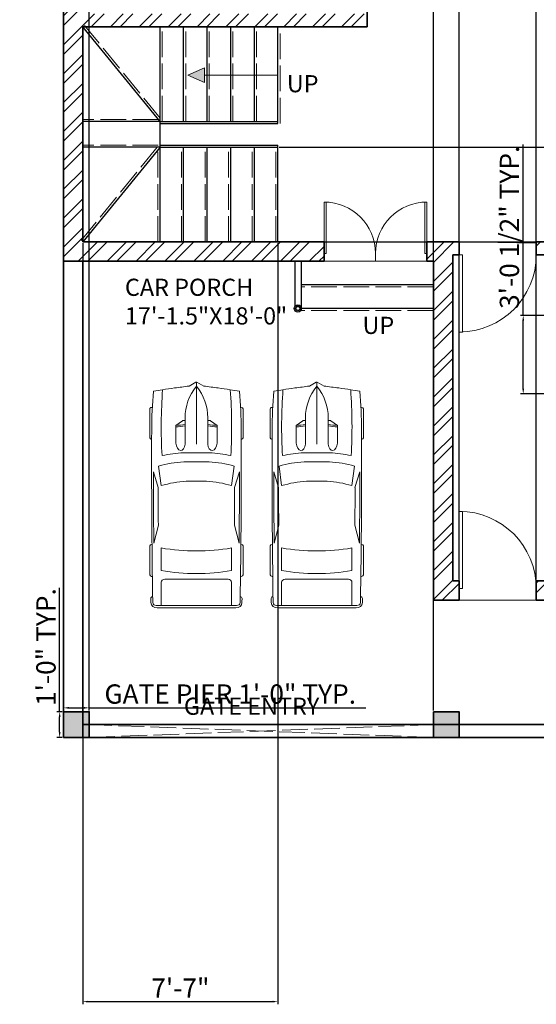
# Model space of a CAD drawing. Units: inches. Extents: x 744 to 1448, y 5126 to 6077.
# Tile 1 of 10: x 784 to 1025, y 5126 to 5585. Entities that reach past the tile are written whole.
import ezdxf

# ---------------------------------------------------------------- set-up
doc = ezdxf.new("R2010")
doc.units = ezdxf.units.IN
doc.linetypes.add('ACAD_ISO02W100', pattern=[15, 12, -3])
for name, color, linetype, lineweight in [('A-ANNO-DIMS', 2, 'Continuous', 18), ('A-ANNO-SYMB', 7, 'Continuous', 18), ('A-ANNO-TEXT', 7, 'Continuous', 18), ('A-AREA-IDEN', 7, 'Continuous', 18), ('A-COLS', 7, 'Continuous', 35), ('A-DOOR', 4, 'Continuous', 18), ('A-FLOR-STRS', 7, 'Continuous', 25), ('A-FLOR-STRS-HIDN', 8, 'ACAD_ISO02W100', 13), ('A-SITE-VEHI', 8, 'Continuous', 13), ('A-WALL', 7, 'Continuous', 35), ('A-WALL-PATT', 252, 'Continuous', 13)]:
    doc.layers.add(name, color=color, linetype=linetype, lineweight=lineweight)
doc.layers.add('A-SITE-GATE', color=244, linetype='ACAD_ISO02W100', lineweight=13, true_color=0x991b1e)
doc.styles.get("Standard").update_dxf_attribs({"font": 'arial.ttf'})
doc.dimstyles.new('ISO-25', dxfattribs={"dimtxt": 9, "dimasz": 2.5, "dimexe": 1.25, "dimexo": 0.625, "dimtad": 1, "dimlunit": 3, "dimtxsty": 'Standard', "dimcen": 2.5, "dimadec": 0, "dimazin": 0, "dimtfac": 1, "dimtmove": 0, "dimatfit": 3, "dimfxl": 1, "dimarcsym": 0})

# ---------------------------------------------------------------- blocks, each defined once
blk = doc.blocks.new('*U5')
for p, q in [((0, 0), (0, 6)), ((40, 0), (40, 6))]:
    blk.add_line(p, q)
blk.add_lwpolyline([(0, 0), (0, -40), (1.75, -40), (1.75, 0)], close=True)
blk.add_arc((0, 0), 40, 270, 0)
blk = doc.blocks.new('*U2')
for p, q in [((0, 0), (0, -6)), ((40, 0), (40, -6))]:
    blk.add_line(p, q)
blk.add_lwpolyline([(0, 0), (0, 40), (1.75, 40), (1.75, 0)], close=True)
blk.add_arc((0, 0), 40, 0, 90)
blk = doc.blocks.new('*U6')
for p, q in [((0, 0), (0, -6)), ((-40, 0), (-40, -6))]:
    blk.add_line(p, q)
blk.add_lwpolyline([(0, 0), (0, 40), (-1.75, 40), (-1.75, 0)], close=True)
blk.add_arc((0, 0), 40, 90, 180)
blk = doc.blocks.new('*U22')
for p, q in [((21.1, 37.41), (21.1, 36.83)), ((46.55, 38.89), (22.35, 38.89)), ((47.8, 37.39), (47.8, 37.41)), ((87.99, 31.87), (74.76, 35.92)), ((134.31, 35.6), (119.29, 31.78)), ((135.45, 37.07), (135.45, 37.41)), ((136.7, 38.89), (160.9, 38.89)), ((162.15, 37.41), (162.15, 36.77)), ((186.47, -33.5), (186.47, 33.5)), ((70.03, 31.54), (86.41, 29.35)), ((138.42, 29.35), (157.25, 29.35)), ((164.52, 26.39), (164.52, -26.39)), ((186.47, 29.35), (167.01, 29.35)), ((188.4, -32.76), (188.4, 32.76)), ((32.27, 11.63), (36.13, 17.17)), ((36.13, 17.17), (50.94, 17.17)), ((29.77, 9.51), (51.68, 9.51)), ((32.12, 9.51), (32.12, 11.15)), ((58.92, -10.77), (58.92, 10.77)), ((66.55, -10.53), (66.55, 10.53)), ((82.74, 8.5), (82.74, -8.5)), ((186.47, -10.53), (186.47, 10.53)), ((3.27, 6.13), (0.1, 0.41)), ((0, 0), (51.68, 0)), ((0.1, -0.41), (3.27, -6.13)), ((29.77, -9.51), (51.68, -9.51)), ((32.12, -9.51), (32.12, -11.15)), ((32.27, -11.63), (36.13, -17.17)), ((36.13, -17.17), (50.94, -17.17)), ((86.41, -29.35), (70.03, -31.54)), ((87.99, -31.87), (74.76, -35.92)), ((134.31, -35.6), (119.29, -31.78)), ((157.25, -29.35), (138.42, -29.35)), ((167.01, -29.35), (186.47, -29.35)), ((21.1, -37.41), (21.1, -36.83)), ((46.55, -38.89), (22.35, -38.89)), ((47.8, -37.39), (47.8, -37.41)), ((135.45, -37.07), (135.45, -37.41)), ((136.7, -38.89), (160.9, -38.89)), ((162.15, -37.41), (162.15, -36.77))]:
    blk.add_line(p, q)
for centre, major_axis, ratio, start_param, end_param in [((266.03, -27.52), (0, 313.31), 0.842304, 1.367076, 1.39176), ((41.19, -490.86), (0, 528.23), 0.842304, 0.00281, 0.075598), ((22.35, 37.41), (0, -1.48), 0.842304, 3.141593, 4.712389), ((64.48, -10555.62), (0, 10593.03), 0.842304, -0.013397, 0.002797), ((46.55, 37.41), (0, 1.48), 0.842304, -1.570796, 0), ((64.48, -10555.62), (0, -10591.55), 0.842304, 3.133765, 3.140441), ((136.7, 37.41), (0, -1.48), 0.842304, 3.141593, 4.712389), ((160.9, 37.41), (0, 1.48), 0.842304, -1.570796, 0), ((180.63, 35.84), (0, 2.22), 0.842304, -0.013017, 1.249894), ((64.48, -10556.36), (0, 10595.31), 0.842304, -0.013397, -0.013017), ((183.98, 33.5), (0, -2.96), 0.842304, 1.570796, 3.128196), ((183.98, 32.76), (0, -5.25), 0.842304, 1.570796, 3.128196), ((259.18, -27.52), (0, -305.3), 0.842304, 4.528606, 4.561838), ((37.47, -593.96), (0, -623.33), 0.842304, 3.096046, 3.200911), ((134.4, 5.39), (0, -89.78), 0.842304, 4.449482, 4.652344), ((135.29, 5.39), (0, 81.77), 0.842304, 1.245306, 1.50788), ((149.6, 2.8), (0, -79.58), 0.842304, 4.372215, 4.640744), ((95.79, -3666.35), (0, -3698.24), 0.842304, 3.134049, 3.144098), ((17.08, 0), (0, 147.02), 0.842304, 4.511394, 4.913384), ((35.91, 0), (0, 147.02), 0.842304, 4.511394, 4.913384), ((167.01, 26.39), (0, 2.96), 0.842304, 0, 1.570796), ((-204.49, 52.4), (0, -250.96), 0.842304, 1.385369, 1.434372), ((13.04, 17.01), (0, 27.42), 0.842304, 4.435146, 4.718221), ((14.2, 17.01), (0, 27.42), 0.842304, 4.435146, 4.718221), ((50.79, 13.34), (6.34, -0.36), 0.603834, -1.395552, 1.581315), ((29.77, -46.66), (0, 56.17), 0.842304, 0, 0.590319), ((32.75, 11.15), (0, 0.74), 0.842304, 0.879714, 1.570796), ((0.62, 0), (0, -0.74), 0.842304, 4.131459, 5.293319), ((-204.49, -52.4), (0, 250.96), 0.842304, -1.434372, -1.385369), ((29.77, 46.66), (0, 56.17), 0.842304, 2.551274, 3.141593), ((32.75, -11.15), (0, -0.74), 0.842304, 4.712389, 5.403472), ((13.04, -17.01), (0, -27.42), 0.842304, 1.564964, 1.848039), ((14.2, -17.01), (0, -27.42), 0.842304, 1.564964, 1.848039), ((134.4, -5.39), (0, -89.78), 0.842304, -1.510751, -1.307889), ((135.29, -5.39), (0, -81.77), 0.842304, -1.50788, -1.245306), ((149.6, -2.8), (0, -79.58), 0.842304, -1.499151, -1.230623), ((259.18, 27.52), (0, 305.3), 0.842304, 1.721348, 1.754579), ((266.03, 27.52), (0, 313.31), 0.842304, 1.749832, 1.774517), ((37.47, 593.96), (0, -623.33), 0.842304, -0.059319, 0.045547), ((95.79, 3666.35), (0, -3698.24), 0.842304, -0.002505, 0.007544), ((167.01, -26.39), (0, -2.96), 0.842304, 4.712389, 6.283185), ((183.98, -32.76), (0, -5.25), 0.842304, 0.013397, 1.570796), ((41.19, 490.86), (0, -528.23), 0.842304, -0.075598, -0.00281), ((22.35, -37.41), (0, 1.48), 0.842304, 1.570796, 3.141593), ((64.48, 10555.62), (0, 10593.03), 0.842304, 3.138796, 3.15499), ((46.55, -37.41), (0, -1.48), 0.842304, 0, 1.570796), ((64.48, 10555.62), (0, -10591.55), 0.842304, 0.001152, 0.007828), ((136.7, -37.41), (0, -1.48), 0.842304, -1.570796, 0), ((160.9, -37.41), (0, 1.48), 0.842304, 3.141593, 4.712389), ((180.63, -35.84), (0, -2.22), 0.842304, -1.249894, 0.013017), ((64.48, 10556.36), (0, 10595.31), 0.842304, 3.15461, 3.15499), ((183.98, -33.5), (0, 2.96), 0.842304, 3.15499, 4.712389)]:
    blk.add_ellipse(centre, major_axis=major_axis, ratio=ratio, start_param=start_param, end_param=end_param)
at = {"extrusion": (0, 0, -1)}
blk.add_ellipse((50.79, -13.34), major_axis=(6.34, 0.36), ratio=0.603834, start_param=-1.395552, end_param=1.581315, dxfattribs=at)
blk = doc.blocks.new('GATE-PIER-12IN')
h = blk.add_hatch(color=256)
h.dxf.hatch_style = 1
h.paths.add_polyline_path([(0, 0), (12, 0), (12, 12), (0, 12)])
blk.add_lwpolyline([(0, 12), (12, 12), (12, 0), (0, 0)], close=True)
blk = doc.blocks.new('*D44')
at = {"layer": 'A-ANNO-DIMS', "color": 0, "lineweight": -2, "transparency": 16777216}
for p, q in [((1019.08, 5447.1), (1019.08, 5526.68)), ((1031.06, 5447.1), (1017.83, 5447.1)), ((1019.08, 5412.94), (1019.08, 5444.6)), ((1031.06, 5410.44), (1017.83, 5410.44))]:
    blk.add_line(p, q, dxfattribs=at)
at = {"layer": 'A-ANNO-DIMS', "color": 0, "transparency": 16777216}
for points in [[(1018.66, 5444.6), (1019.5, 5444.6), (1019.08, 5447.1)], [(1018.66, 5412.94), (1019.5, 5412.94), (1019.08, 5410.44)]]:
    blk.add_solid(points, dxfattribs=at)
at = {"layer": 'Defpoints', "color": 0, "transparency": 16777216}
for p in [(1019.08, 5447.1), (1031.68, 5447.1), (1031.68, 5410.44)]:
    blk.add_point(p, dxfattribs=at)
at = {"layer": 'A-ANNO-DIMS', "color": 0, "transparency": 16777216, "insert": (1013.8, 5488.14), "char_height": 9, "attachment_point": 5, "rotation": 90}
blk.add_mtext('3\'-0 1/2" TYP.', dxfattribs=at)
blk = doc.blocks.new('*D53')
at = {"layer": 'A-ANNO-DIMS', "color": 0, "lineweight": -2, "transparency": 16777216}
for p, q in [((804.68, 5262.94), (804.68, 5265.37)), ((816.68, 5262.94), (816.68, 5265.37)), ((807.18, 5264.12), (814.18, 5264.12)), ((816.68, 5264.12), (945.71, 5264.12))]:
    blk.add_line(p, q, dxfattribs=at)
at = {"layer": 'A-ANNO-DIMS', "color": 0, "transparency": 16777216}
for points in [[(807.18, 5264.53), (807.18, 5263.7), (804.68, 5264.12)], [(814.18, 5264.53), (814.18, 5263.7), (816.68, 5264.12)]]:
    blk.add_solid(points, dxfattribs=at)
at = {"layer": 'Defpoints', "color": 0, "transparency": 16777216}
for p in [(804.68, 5262.32), (816.68, 5264.12), (816.68, 5262.32)]:
    blk.add_point(p, dxfattribs=at)
at = {"layer": 'A-ANNO-DIMS', "color": 0, "transparency": 16777216, "insert": (882.45, 5269.39), "char_height": 9, "attachment_point": 5}
blk.add_mtext('GATE PIER 1\'-0" TYP.', dxfattribs=at)
blk = doc.blocks.new('*D54')
at = {"layer": 'A-ANNO-DIMS', "color": 0, "lineweight": -2, "transparency": 16777216}
for p, q in [((802.88, 5262.32), (802.88, 5320.08)), ((804.06, 5262.32), (801.63, 5262.32)), ((802.88, 5252.82), (802.88, 5259.82)), ((804.06, 5250.32), (801.63, 5250.32))]:
    blk.add_line(p, q, dxfattribs=at)
at = {"layer": 'A-ANNO-DIMS', "color": 0, "transparency": 16777216}
for points in [[(802.47, 5259.82), (803.3, 5259.82), (802.88, 5262.32)], [(802.47, 5252.82), (803.3, 5252.82), (802.88, 5250.32)]]:
    blk.add_solid(points, dxfattribs=at)
at = {"layer": 'Defpoints', "color": 0, "transparency": 16777216}
for p in [(802.88, 5262.32), (804.68, 5262.32), (804.68, 5250.32)]:
    blk.add_point(p, dxfattribs=at)
at = {"layer": 'A-ANNO-DIMS', "color": 0, "transparency": 16777216, "insert": (797.66, 5292.45), "char_height": 9, "attachment_point": 5, "rotation": 90}
blk.add_mtext('1\'-0" TYP.', dxfattribs=at)
blk = doc.blocks.new('*D55')
at = {"layer": 'A-ANNO-DIMS', "color": 0, "lineweight": -2, "transparency": 16777216}
for p, q in [((989.18, 5323.94), (989.18, 6059.61)), ((1025.18, 5323.94), (1025.18, 6059.61)), ((991.68, 6058.36), (1022.68, 6058.36))]:
    blk.add_line(p, q, dxfattribs=at)
at = {"layer": 'A-ANNO-DIMS', "color": 0, "transparency": 16777216}
for points in [[(991.68, 6058.78), (991.68, 6057.95), (989.18, 6058.36)], [(1022.68, 6058.78), (1022.68, 6057.95), (1025.18, 6058.36)]]:
    blk.add_solid(points, dxfattribs=at)
at = {"layer": 'Defpoints', "color": 0, "transparency": 16777216}
for p in [(1025.18, 6058.36), (989.18, 5323.32), (1025.18, 5323.32)]:
    blk.add_point(p, dxfattribs=at)
at = {"layer": 'A-ANNO-DIMS', "color": 0, "transparency": 16777216, "insert": (1007.18, 6063.59), "char_height": 9, "attachment_point": 5}
blk.add_mtext('3\'-0"', dxfattribs=at)
blk = doc.blocks.new('*D60')
at = {"layer": 'A-ANNO-DIMS', "color": 0, "lineweight": -2, "transparency": 16777216}
for p, q in [((813.68, 5480.69), (813.68, 5125.91)), ((904.68, 5480.69), (904.68, 5125.91)), ((816.18, 5127.16), (902.18, 5127.16))]:
    blk.add_line(p, q, dxfattribs=at)
at = {"layer": 'A-ANNO-DIMS', "color": 0, "transparency": 16777216}
for points in [[(816.18, 5127.58), (816.18, 5126.75), (813.68, 5127.16)], [(902.18, 5127.58), (902.18, 5126.75), (904.68, 5127.16)]]:
    blk.add_solid(points, dxfattribs=at)
at = {"layer": 'Defpoints', "color": 0, "transparency": 16777216}
for p in [(813.68, 5481.32), (904.68, 5481.32), (904.68, 5127.16)]:
    blk.add_point(p, dxfattribs=at)
at = {"layer": 'A-ANNO-DIMS', "color": 0, "transparency": 16777216, "insert": (859.18, 5132.29), "char_height": 9, "attachment_point": 5}
blk.add_mtext('7\'-7"', dxfattribs=at)
blk = doc.blocks.new('*D61')
at = {"layer": 'A-ANNO-DIMS', "color": 0, "lineweight": -2, "transparency": 16777216}
for p, q in [((905.31, 5525.47), (1415.33, 5525.47)), ((1414.08, 5483.82), (1414.08, 5522.97)), ((905.31, 5481.32), (1415.33, 5481.32))]:
    blk.add_line(p, q, dxfattribs=at)
at = {"layer": 'A-ANNO-DIMS', "color": 0, "transparency": 16777216}
for points in [[(1413.67, 5522.97), (1414.5, 5522.97), (1414.08, 5525.47)], [(1413.67, 5483.82), (1414.5, 5483.82), (1414.08, 5481.32)]]:
    blk.add_solid(points, dxfattribs=at)
at = {"layer": 'Defpoints', "color": 0, "transparency": 16777216}
for p in [(904.68, 5525.47), (1414.08, 5525.47), (904.68, 5481.32)]:
    blk.add_point(p, dxfattribs=at)
at = {"layer": 'A-ANNO-DIMS', "color": 0, "transparency": 16777216, "insert": (1408.86, 5503.39), "char_height": 9, "attachment_point": 5, "rotation": 90}
blk.add_mtext('3\'-8"', dxfattribs=at)
blk = doc.blocks.new('*D62')
at = {"layer": 'A-ANNO-DIMS', "color": 0, "lineweight": -2, "transparency": 16777216}
for p, q in [((816.68, 5262.94), (816.68, 6059.61)), ((977.18, 5262.94), (977.18, 6059.61)), ((819.18, 6058.36), (974.68, 6058.36))]:
    blk.add_line(p, q, dxfattribs=at)
at = {"layer": 'A-ANNO-DIMS', "color": 0, "transparency": 16777216}
for points in [[(819.18, 6058.78), (819.18, 6057.95), (816.68, 6058.36)], [(974.68, 6058.78), (974.68, 6057.95), (977.18, 6058.36)]]:
    blk.add_solid(points, dxfattribs=at)
at = {"layer": 'Defpoints', "color": 0, "transparency": 16777216}
for p in [(977.18, 6058.36), (816.68, 5262.32), (977.18, 5262.32)]:
    blk.add_point(p, dxfattribs=at)
at = {"layer": 'A-ANNO-DIMS', "color": 0, "transparency": 16777216, "insert": (896.93, 6063.64), "char_height": 9, "attachment_point": 5}
blk.add_mtext('13\'-4 1/2"', dxfattribs=at)

msp = doc.modelspace()

# ---------------------------------------------------------------- hatches: boundary and pattern name
at = {"layer": 'A-ANNO-SYMB'}
h = msp.add_hatch(color=256, dxfattribs=at)
h.dxf.hatch_style = 1
h.paths.add_polyline_path([(870.507, 5562.481), (862.658, 5559.091), (870.507, 5555.7)])
at = {"layer": 'A-WALL-PATT'}
h = msp.add_hatch(dxfattribs=at)
h.set_pattern_fill('ANSI32', color=256)
h.paths.add_polyline_path([(813.684, 5750.816), (876.684, 5750.816), (876.684, 5756.816), (813.684, 5756.816), (813.684, 5812.816), (909.684, 5812.816), (909.684, 5795.316), (915.684, 5795.316), (915.684, 5812.816), (1209.684, 5812.816), (1209.684, 5795.316), (1215.684, 5795.316), (1215.684, 5812.816), (1311.684, 5812.816), (1311.684, 5756.816), (1248.684, 5756.816), (1248.684, 5750.816), (1311.684, 5750.816), (1311.684, 5570.816), (1179.044, 5570.816), (1179.044, 5564.816), (1311.684, 5564.816), (1311.684, 5383.316), (1260.684, 5383.316), (1260.684, 5377.316), (1311.684, 5377.316), (1311.684, 5320.316), (1227.684, 5320.316), (1227.684, 5333.816), (1221.684, 5333.816), (1221.684, 5314.316), (1320.684, 5314.316), (1320.684, 5821.816), (804.684, 5821.816), (804.684, 5472.316), (926.184, 5472.316), (926.184, 5481.316), (813.684, 5481.316), (813.684, 5581.616), (946.284, 5581.616), (946.284, 5587.616), (813.684, 5587.616)])
h.paths.add_polyline_path([(1155.684, 5525.816), (1149.684, 5525.816), (1149.684, 5481.316), (1025.184, 5481.316), (1025.184, 5475.316), (1146.684, 5475.316), (1146.684, 5323.316), (1118.788, 5323.316), (1118.788, 5314.316), (1146.684, 5314.316), (1155.684, 5314.316), (1155.684, 5374.316), (1170.35, 5374.316), (1170.35, 5383.316), (1155.684, 5383.316)], flags=17)
h.paths.add_polyline_path([(1230.684, 5383.316), (1213.35, 5383.316), (1213.35, 5374.316), (1221.684, 5374.316), (1221.684, 5363.816), (1226.184, 5363.816), (1227.684, 5363.816), (1227.684, 5377.316), (1230.684, 5377.316)], flags=17)
h.paths.add_polyline_path([(1185.684, 5671.816), (1155.684, 5671.816), (1155.684, 5750.816), (1161.575, 5750.816), (1161.575, 5756.816), (1157.542, 5756.816), (1157.847, 5756.715), (1155.79, 5756.816), (1149.684, 5756.816), (1149.684, 5750.816), (1149.684, 5671.816), (1121.684, 5671.816), (1121.684, 5665.816), (1179.684, 5665.816), (1179.684, 5609.816), (1185.684, 5609.816)], flags=17)
h.paths.add_polyline_path([(1003.684, 5671.816), (975.684, 5671.816), (975.684, 5750.816), (975.684, 5756.816), (965.205, 5756.816), (965.205, 5750.816), (969.684, 5750.816), (969.684, 5671.816), (939.684, 5671.816), (939.684, 5626.616), (945.684, 5626.616), (945.684, 5665.816), (1003.684, 5665.816)], flags=17)
h.paths.add_polyline_path([(915.684, 5774.316), (909.684, 5774.316), (909.684, 5756.816), (906.684, 5756.816), (906.684, 5752.316), (906.684, 5750.816), (922.205, 5750.816), (922.205, 5756.816), (915.684, 5756.816)], flags=17)
h.paths.add_polyline_path([(1215.684, 5774.316), (1209.684, 5774.316), (1209.684, 5756.816), (1204.575, 5756.816), (1204.575, 5750.816), (1218.684, 5750.816), (1218.684, 5756.816), (1215.684, 5756.816)], flags=17)
h.paths.add_polyline_path([(1063.788, 5323.316), (1025.184, 5323.316), (1025.184, 5314.316), (1063.788, 5314.316)])
h.paths.add_polyline_path([(986.184, 5475.316), (989.184, 5475.316), (989.184, 5481.316), (974.184, 5481.316), (974.184, 5475.916), (974.184, 5472.316), (977.184, 5472.316), (977.184, 5314.316), (989.184, 5314.316), (989.184, 5319.716), (989.184, 5323.316), (986.184, 5323.316)])

# ---------------------------------------------------------------- linework, layer by layer
at = {"layer": 'A-ANNO-SYMB'}
msp.add_line((904.684, 5559.091), (870.507, 5559.091), dxfattribs=at)
msp.add_lwpolyline([(862.658, 5559.091), (870.507, 5555.7), (870.507, 5562.481)], close=True, dxfattribs=at)
at = {"layer": 'A-DOOR'}
for p, q in [((989.184, 5481.316), (1025.184, 5480.716)), ((974.184, 5472.316), (926.184, 5472.316)), ((1025.184, 5314.316), (989.184, 5314.316))]:
    msp.add_line(p, q, dxfattribs=at)
at = {"layer": 'A-FLOR-STRS'}
for p, q in [((849.684, 5537.466), (813.684, 5581.616)), ((849.684, 5481.316), (849.684, 5581.616)), ((860.684, 5537.466), (860.684, 5581.616)), ((871.684, 5537.466), (871.684, 5581.616)), ((882.684, 5537.466), (882.684, 5581.616)), ((893.684, 5537.466), (893.684, 5581.616)), ((904.684, 5536.566), (904.684, 5581.616)), ((849.684, 5537.466), (813.684, 5537.466)), ((849.684, 5537.466), (904.684, 5537.466)), ((849.684, 5536.566), (904.684, 5536.566)), ((849.684, 5525.466), (813.684, 5525.466)), ((849.684, 5525.466), (813.684, 5481.316)), ((849.684, 5526.366), (904.684, 5526.366)), ((849.684, 5525.466), (904.684, 5525.466)), ((860.684, 5481.316), (860.684, 5525.466)), ((871.684, 5481.316), (871.684, 5525.466)), ((882.684, 5481.316), (882.684, 5525.466)), ((893.684, 5481.316), (893.684, 5525.466)), ((904.684, 5481.316), (904.684, 5526.366)), ((912.511, 5472.316), (912.511, 5451.149)), ((915.511, 5472.316), (915.511, 5451.125)), ((977.184, 5461.316), (915.511, 5461.316)), ((977.184, 5450.316), (915.714, 5450.316))]:
    msp.add_line(p, q, dxfattribs=at)
for radius in [1.71, 1.11, 0.91]:
    msp.add_circle((914.004, 5450.316), radius, dxfattribs=at)
at = {"layer": 'A-FLOR-STRS-HIDN'}
for p, q in [((849.684, 5539.048), (814.459, 5582.248)), ((850.684, 5537.466), (850.684, 5581.616)), ((861.684, 5537.466), (861.684, 5581.616)), ((872.684, 5537.466), (872.684, 5581.616)), ((883.684, 5537.466), (883.684, 5581.616)), ((894.684, 5537.466), (894.684, 5581.616)), ((905.684, 5536.566), (905.684, 5581.616)), ((848.869, 5538.466), (813.684, 5538.466)), ((848.394, 5525.466), (812.909, 5481.948)), ((848.869, 5526.466), (813.684, 5526.466)), ((848.684, 5481.316), (848.684, 5524.239)), ((859.684, 5481.316), (859.684, 5525.466)), ((870.684, 5481.316), (870.684, 5525.466)), ((881.684, 5481.316), (881.684, 5525.466)), ((892.684, 5481.316), (892.684, 5525.466)), ((903.684, 5481.316), (903.684, 5525.466)), ((977.184, 5460.316), (915.511, 5460.316)), ((977.184, 5449.316), (915.714, 5449.316))]:
    msp.add_line(p, q, dxfattribs=at)
at = {"layer": 'A-SITE-GATE'}
for p, q in [((816.684, 5250.316), (977.184, 5256.316)), ((977.184, 5250.316), (816.684, 5256.316))]:
    msp.add_line(p, q, dxfattribs=at)
at = {"layer": 'A-WALL'}
for p, q in [((804.684, 5250.316), (804.684, 5821.816)), ((946.284, 5590.616), (946.284, 5581.616)), ((813.684, 5581.616), (946.284, 5581.616)), ((813.684, 5481.316), (813.684, 5581.616)), ((813.684, 5481.316), (926.184, 5481.316)), ((926.184, 5472.316), (926.184, 5481.316)), ((974.184, 5472.316), (974.184, 5481.316)), ((974.184, 5481.316), (989.184, 5481.316)), ((989.184, 5475.316), (989.184, 5481.316)), ((1025.184, 5475.316), (1025.184, 5481.316)), ((1025.184, 5481.316), (1149.684, 5481.316)), ((804.684, 5472.316), (926.184, 5472.316)), ((813.684, 5250.316), (813.684, 5472.316)), ((974.184, 5472.316), (977.184, 5472.316)), ((977.184, 5314.316), (977.184, 5472.316)), ((986.184, 5323.316), (986.184, 5475.316)), ((986.184, 5475.316), (989.184, 5475.316)), ((1025.184, 5475.316), (1146.684, 5475.316)), ((986.184, 5323.316), (989.184, 5323.316)), ((989.184, 5323.316), (989.184, 5314.316)), ((1025.184, 5323.316), (1025.184, 5314.316)), ((1025.184, 5323.316), (1146.684, 5323.316)), ((977.184, 5314.316), (989.184, 5314.316)), ((1025.184, 5314.316), (1146.684, 5314.316)), ((813.684, 5256.316), (1311.684, 5256.316)), ((804.684, 5250.316), (1320.684, 5250.316))]:
    msp.add_line(p, q, dxfattribs=at)

# ---------------------------------------------------------------- block references
at = {"layer": 'A-COLS'}
for p in [(804.684, 5250.316), (977.184, 5250.316)]:
    msp.add_blockref('GATE-PIER-12IN', p, dxfattribs=at)
at = {"layer": 'A-DOOR'}
for name, p, xscale, yscale, zscale in [('*U2', (926.184, 5475.916), 0.6, 0.6, 0.6), ('*U6', (974.184, 5475.916), 0.6, 0.6, 0.6), ('*U5', (989.184, 5475.316), 0.9, 0.9, 0.9), ('*U2', (989.184, 5319.716), 0.9, 0.9, 0.9)]:
    msp.add_blockref(name, p, dxfattribs=dict(at, xscale=xscale, yscale=yscale, zscale=zscale))
at = {"layer": 'A-SITE-VEHI', "xscale": 0.5587074559707127, "yscale": 0.5587074559707127, "zscale": 0.5587074559707127, "rotation": 270}
for p in [(866.678, 5415.989), (922.818, 5415.989)]:
    msp.add_blockref('*U22', p, dxfattribs=at)

# ---------------------------------------------------------------- texts
at = {"layer": 'A-ANNO-TEXT', "char_height": 8, "attachment_point": 1}
for s, width, insert in [('UP', 17.2756, (908.841, 5559.091)), ('UP', 17.2756, (944.134, 5446.422)), ('GATE ENTRY', 73.54978, (860.827, 5268.865))]:
    msp.add_mtext_dynamic_manual_height_columns(s, width=width, gutter_width=12.5, heights=[0], dxfattribs=dict(at, insert=insert))
at = {"layer": 'A-AREA-IDEN', "insert": (833.324, 5464.179), "char_height": 8, "attachment_point": 1}
msp.add_mtext_dynamic_manual_height_columns('CAR PORCH\\P17\'-1.5"X18\'-0"', width=70.44947, gutter_width=12.5, heights=[0], dxfattribs=at)

# ---------------------------------------------------------------- dimensions: what is measured, and where the dimension line sits
at = {"layer": 'A-ANNO-DIMS'}
for base, p1, p2, picture, middle in [((977.184, 6058.363), (816.684, 5262.316), (977.184, 5262.316), '*D62', (896.934, 6063.645)), ((1025.184, 6058.363), (989.184, 5323.316), (1025.184, 5323.316), '*D55', (1007.184, 6063.586)), ((904.684, 5127.162), (813.684, 5481.316), (904.684, 5481.316), '*D60', (859.184, 5132.287))]:
    dim = msp.add_linear_dim(base=base, p1=p1, p2=p2, dimstyle='ISO-25', override={"dimdec": 1, "dimlfac": 1, "dimrnd": 0, "dimzin": 1, "dimdsep": 46, "dimlunit": 4, "dimfrac": 2}, dxfattribs=at)
    dim.commit()
    dim.dimension.update_dxf_attribs({"geometry": picture, "text_midpoint": middle})
for base, p1, p2, picture, middle in [((1019.08, 5447.103), (1031.68, 5410.436), (1031.68, 5447.103), '*D44', (1013.799, 5488.14)), ((802.884, 5262.316), (804.684, 5250.316), (804.684, 5262.316), '*D54', (797.664, 5292.447))]:
    dim = msp.add_linear_dim(base=base, p1=p1, p2=p2, angle=90, text='<> TYP.', dimstyle='ISO-25', override={"dimdec": 1, "dimlfac": 1, "dimrnd": 0, "dimzin": 1, "dimdsep": 46, "dimlunit": 4, "dimfrac": 2}, dxfattribs=at)
    dim.commit()
    dim.dimension.update_dxf_attribs({"geometry": picture, "text_midpoint": middle})
dim = msp.add_linear_dim(base=(1414.084316, 5525.465662), p1=(904.684316, 5481.315662), p2=(904.684316, 5525.465662), angle=90, dimstyle='ISO-25', override={"dimdec": 1, "dimlfac": 1, "dimrnd": 0, "dimzin": 1, "dimdsep": 46, "dimlunit": 4, "dimfrac": 2}, dxfattribs=at)
dim.commit()
dim.dimension.update_dxf_attribs({"geometry": '*D61', "text_midpoint": (1408.861089533, 5503.390662)})
dim = msp.add_linear_dim(base=(816.684, 5264.116), p1=(804.684, 5262.316), p2=(816.684, 5262.316), text='GATE PIER <> TYP.', dimstyle='ISO-25', override={"dimdec": 1, "dimlfac": 1, "dimrnd": 0, "dimzin": 1, "dimdsep": 46, "dimlunit": 4, "dimfrac": 2}, dxfattribs=at)
dim.commit()
dim.dimension.update_dxf_attribs({"geometry": '*D53', "text_midpoint": (882.447, 5269.394)})

doc.saveas('drawing.dxf')
